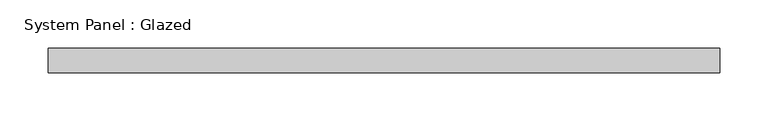
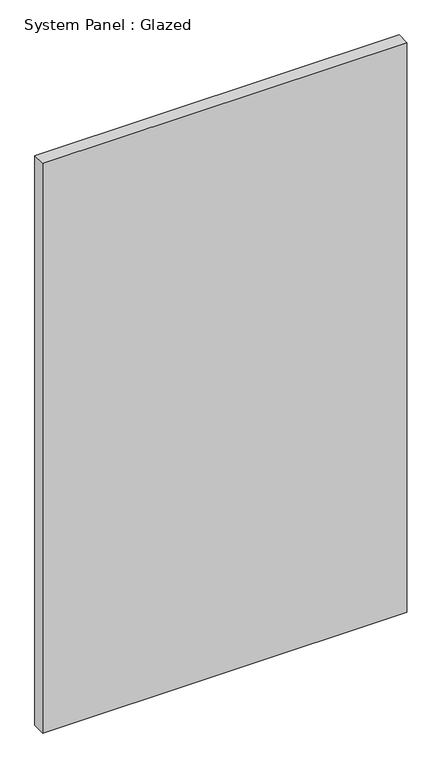
"""IFC4 building model written with IfcOpenShell, lengths in millimetres: plate geometry, System Panel : Glazed."""

from ifc_helpers import new_model, si_unit, origin, origin_with_axes, place, context, project, spatial, polyline, outline, extrude, source, transform, mapped, element, save


def system_panel_glazed_7b5ce646(model_context):
    return source(origin(), model_context, "Body", "SweptSolid", [
        extrude(outline(polyline([(349.25, 19.05), (-349.25, 19.05), (-349.25, 44.45), (349.25, 44.45), (349.25, 19.05)])), origin_with_axes(), (0.0, 0.0, 1.0), 1155.7),
    ])


if __name__ == "__main__":
    model = new_model("IFC4")
    model_context = context("Model", 3, world=origin())
    ifc_project = project(units=[si_unit("LENGTHUNIT", "METRE", prefix="MILLI")], contexts=[model_context])
    site = spatial("IfcSite", under=ifc_project)
    building = spatial("IfcBuilding", under=site)
    placement = place(None, origin())
    system_panel_glazed_shape = system_panel_glazed_7b5ce646(model_context)
    element("IfcPlate", 1, ObjectType="System Panel : Glazed", at=placement, inside=building, context=model_context, shape_type="MappedRepresentation", body=[
        mapped(system_panel_glazed_shape, transform((0.0, 0.0, 0.0), x_axis=(1.0, 0.0, 0.0), y_axis=(0.0, 1.0, 0.0), z_axis=(0.0, 0.0, 1.0))),
    ])
    save(model, "model.ifc")

# Revit data of these elements
# Type "System Panel : Glazed"
#   Construction Type Id = "GSP4R"
#   Analytic Construction = "1/8 in Pilkington single glazing"
#   Visual Light Transmittance = 0.9
#   Solar Heat Gain Coefficient = 0.86
#   Heat Transfer Coefficient (U) = 1.18115 BTU/(h·ft²·°F)
# Element 1 (IfcPlate, "System Panel : Glazed")
#   Materials on its faces: "Glass"
# Materials
#   "Glass": class "Glass", colour RGB 0 128 192, transparency 0.75, Description = "Soda Lime Glass", Cost = 0
